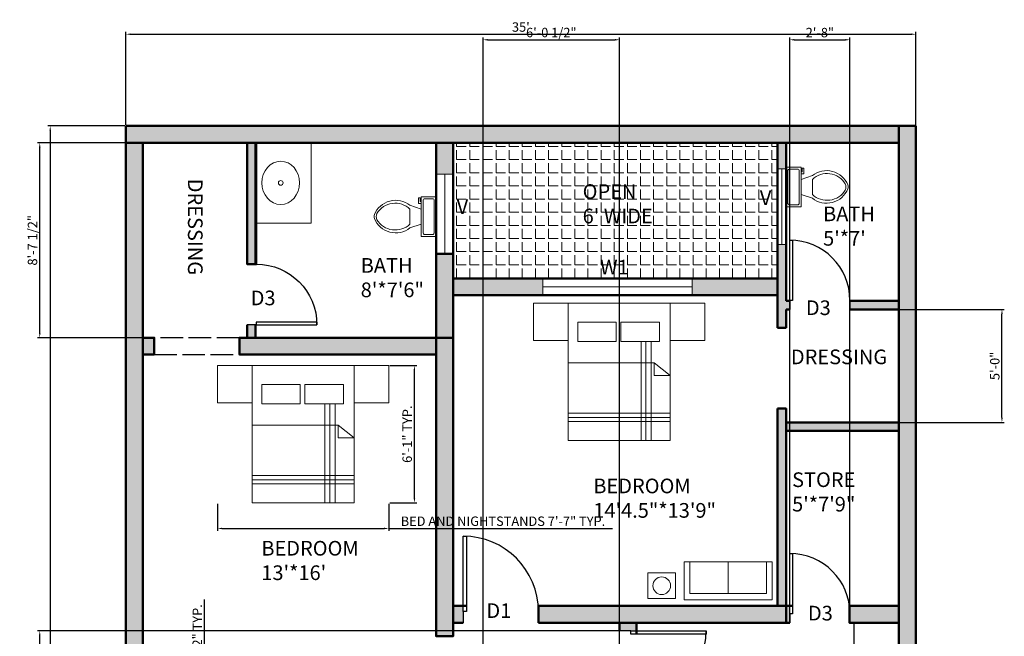
# Model space of a CAD drawing. Units: inches. Extents: x 2191 to 2715, y 2502 to 3448.
# Tile 3 of 3: x 2191 to 2715, y 3120 to 3448. Entities that reach past the tile are written whole.
import ezdxf

# ---------------------------------------------------------------- set-up
doc = ezdxf.new("R2010")
doc.units = ezdxf.units.IN
doc.linetypes.add('ACAD_ISO02W100', pattern=[15, 12, -3])
for name, color, linetype, lineweight in [('A-ANNO-DIMS', 2, 'Continuous', 18), ('A-AREA-IDEN', 130, 'Continuous', 25), ('A-FLOR-CASE', 9, 'Continuous', 25), ('A-FLOR-FIXT', 8, 'Continuous', 18), ('A-FLOR-PATT', 9, 'Continuous', 13), ('A-WALL-OVHD', 150, 'ACAD_ISO02W100', 25), ('A-WALL-PATT', 150, 'Continuous', 13), ('DOOR', 52, 'Continuous', 25), ('FUR', 140, 'Continuous', 18), ('TEXT', 130, 'Continuous', 18), ('WALL', 150, 'Continuous', 50), ('WIN', 210, 'Continuous', 18)]:
    doc.layers.add(name, color=color, linetype=linetype, lineweight=lineweight)
doc.styles.get("Standard").update_dxf_attribs({"font": 'arial.ttf'})
doc.dimstyles.new('ISO-25', dxfattribs={"dimtxt": 5, "dimasz": 2.5, "dimexe": 1.25, "dimexo": 0.625, "dimtad": 1, "dimdec": 0, "dimlunit": 4, "dimtxsty": 'Standard', "dimcen": 2.5, "dimadec": 0, "dimazin": 0, "dimtfac": 1, "dimtdec": 0, "dimtmove": 0, "dimatfit": 3, "dimfxl": 1, "dimarcsym": 0})

# ---------------------------------------------------------------- blocks, each defined once
blk = doc.blocks.new('*U2')
for p, q in [((0, 0), (0, -6)), ((40, 0), (40, -6))]:
    blk.add_line(p, q)
blk.add_lwpolyline([(0, 0), (0, 40), (1.75, 40), (1.75, 0)], close=True)
blk.add_arc((0, 0), 40, 0, 90)
blk = doc.blocks.new('*U4')
for p, q in [((9.5, -6), (9.5, -2)), ((-10, -8.5), (-8, -8.5)), ((-10, -9.5), (-10, -8.5)), ((-7, -9.5), (-10, -9.5)), ((-8, -8.5), (-8, -8)), ((-7, -8), (-7, -9.5)), ((-4, -8), (-6, -14)), ((4, -8), (6, -14)), ((4, -14), (-4, -14))]:
    blk.add_line(p, q)
blk.add_lwpolyline([(10.5, -8), (10.5, 0), (-10.5, 0), (-10.5, -8)], close=True)
for points in [[(-9.5, -2), (-9.5, -6)], [(8.5, -1), (-8.5, -1)], [(-8.5, -7), (8.5, -7)]]:
    blk.add_lwpolyline(points)
for centre, radius, start, end in [((-8.62, -1.88), 0.884, 81.8699, 188.1301), ((8.62, -1.88), 0.884, 351.8699, 98.1301), ((-8.62, -6.12), 0.884, 171.8699, 278.1301), ((8.62, -6.12), 0.884, 261.8699, 8.1301), ((3.52, -21.58), 12.17, 141.4691, 247.9714), ((4.2, -21.82), 11.33, 136.3677, 238.9468), ((-3.52, -21.58), 12.17, 292.0284, 38.5307), ((-4.2, -21.82), 11.33, 301.053, 43.6321), ((0, -27.88), 4, 245.7318, 294.2682), ((0, -29), 4, 254.8605, 285.1395)]:
    blk.add_arc(centre, radius, start, end)
blk = doc.blocks.new('*D8')
at = {"layer": 'A-ANNO-DIMS', "color": 0, "lineweight": -2, "transparency": 16777216}
for p, q in [((2247.96, 3392.28), (2247.96, 3441.65)), ((2250.46, 3440.4), (2665.46, 3440.4)), ((2667.96, 3392.28), (2667.96, 3441.65))]:
    blk.add_line(p, q, dxfattribs=at)
at = {"layer": 'A-ANNO-DIMS', "color": 0, "lineweight": 100, "transparency": 16777216}
for points in [[(2250.46, 3440.82), (2250.46, 3439.99), (2247.96, 3440.4)], [(2665.46, 3440.82), (2665.46, 3439.99), (2667.96, 3440.4)]]:
    blk.add_solid(points, dxfattribs=at)
at = {"layer": 'Defpoints', "color": 0, "lineweight": 100, "transparency": 16777216}
for p in [(2667.96, 3440.4), (2247.96, 3391.65), (2667.96, 3391.65)]:
    blk.add_point(p, dxfattribs=at)
at = {"layer": 'A-ANNO-DIMS', "color": 0, "transparency": 16777216, "insert": (2457.96, 3443.58), "char_height": 5, "attachment_point": 5}
blk.add_mtext("35'", dxfattribs=at)
blk = doc.blocks.new('*D9')
at = {"layer": 'A-ANNO-DIMS', "color": 0, "lineweight": -2, "transparency": 16777216}
for p, q in [((2247.34, 3391.65), (2206.49, 3391.65)), ((2207.74, 3389.15), (2207.74, 2554.15)), ((2247.34, 2551.65), (2206.49, 2551.65))]:
    blk.add_line(p, q, dxfattribs=at)
at = {"layer": 'A-ANNO-DIMS', "color": 0, "lineweight": 100, "transparency": 16777216}
for points in [[(2207.32, 3389.15), (2208.15, 3389.15), (2207.74, 3391.65)], [(2207.32, 2554.15), (2208.15, 2554.15), (2207.74, 2551.65)]]:
    blk.add_solid(points, dxfattribs=at)
at = {"layer": 'Defpoints', "color": 0, "lineweight": 100, "transparency": 16777216}
for p in [(2247.96, 3391.65), (2207.74, 2551.65), (2247.96, 2551.65)]:
    blk.add_point(p, dxfattribs=at)
at = {"layer": 'A-ANNO-DIMS', "color": 0, "transparency": 16777216, "insert": (2204.56, 2971.65), "char_height": 5, "attachment_point": 5, "rotation": 90}
blk.add_mtext("70'", dxfattribs=at)
blk = doc.blocks.new('BED-DOUBLE-WITH-NIGHTSTANDS')
for p, q in [((57.17, 52.58), (57.17, 0)), ((59.74, 52.58), (59.74, 0)), ((62.55, 52.58), (62.55, 0)), ((18.38, 41.27), (64.16, 41.27)), ((64.16, 41.27), (64.16, 34.46)), ((72.67, 34.46), (64.16, 41.27)), ((64.16, 34.46), (72.67, 34.46)), ((72.67, 14.44), (18.38, 14.44)), ((72.67, 12.22), (18.38, 12.22)), ((72.67, 10), (18.38, 10))]:
    blk.add_line(p, q)
for points in [[(0, 72.89), (18.38, 72.89), (18.38, 53.14), (0, 53.14)], [(18.38, 72.89), (72.67, 72.89), (72.67, 0), (18.38, 0)], [(72.67, 72.89), (91.05, 72.89), (91.05, 53.14), (72.67, 53.14)], [(46.51, 62.88), (66.93, 62.88), (66.93, 52.58), (46.51, 52.58)], [(23.55, 62.79), (43.97, 62.79), (43.97, 52.5), (23.55, 52.5)]]:
    blk.add_lwpolyline(points, close=True)
blk = doc.blocks.new('SOFA-TWO-SEAT')
for p, q in [((3.01, 20.24), (0, 20.24)), ((0, 20.24), (0, 0)), ((23.39, 20.24), (23.39, 3.45)), ((43.77, 20.24), (46.65, 20.24)), ((46.65, 20.24), (46.65, 20.24)), ((46.65, 20.24), (46.65, 0)), ((0, 0), (46.65, 0))]:
    blk.add_line(p, q)
blk.add_lwpolyline([(43.77, 3.45), (3.01, 3.45), (3.01, 20.24), (43.77, 20.24)], close=True)
blk = doc.blocks.new('TABLE-END-ROUND-ON-SQUARE')
blk.add_lwpolyline([(14.61, 0), (0, 0), (0, 13.55), (14.61, 13.55)], close=True)
blk.add_circle((7.31, 6.78), 4.68)
blk = doc.blocks.new('*D20')
at = {"layer": 'A-ANNO-DIMS', "color": 0, "lineweight": -2, "transparency": 16777216}
for p, q in [((2296.65, 3190.79), (2296.65, 3176.51)), ((2387.7, 3190.79), (2387.7, 3176.51)), ((2299.15, 3177.76), (2385.2, 3177.76)), ((2387.7, 3177.76), (2506.7, 3177.76))]:
    blk.add_line(p, q, dxfattribs=at)
at = {"layer": 'A-ANNO-DIMS', "color": 0, "lineweight": 100, "transparency": 16777216}
for points in [[(2299.15, 3178.17), (2299.15, 3177.34), (2296.65, 3177.76)], [(2385.2, 3178.17), (2385.2, 3177.34), (2387.7, 3177.76)]]:
    blk.add_solid(points, dxfattribs=at)
at = {"layer": 'Defpoints', "color": 0, "lineweight": 100, "transparency": 16777216}
for p in [(2296.65, 3191.41), (2387.7, 3191.41), (2387.7, 3177.76)]:
    blk.add_point(p, dxfattribs=at)
at = {"layer": 'A-ANNO-DIMS', "color": 0, "transparency": 16777216, "insert": (2448.45, 3180.97), "char_height": 5, "attachment_point": 5}
blk.add_mtext('BED AND NIGHTSTANDS 7\'-7" TYP.', dxfattribs=at)
blk = doc.blocks.new('*D21')
at = {"layer": 'A-ANNO-DIMS', "color": 0, "lineweight": -2, "transparency": 16777216}
for p, q in [((2388.33, 3264.3), (2402.61, 3264.3)), ((2401.36, 3193.91), (2401.36, 3261.8)), ((2388.33, 3191.41), (2402.61, 3191.41))]:
    blk.add_line(p, q, dxfattribs=at)
at = {"layer": 'A-ANNO-DIMS', "color": 0, "lineweight": 100, "transparency": 16777216}
for points in [[(2400.94, 3261.8), (2401.78, 3261.8), (2401.36, 3264.3)], [(2400.94, 3193.91), (2401.78, 3193.91), (2401.36, 3191.41)]]:
    blk.add_solid(points, dxfattribs=at)
at = {"layer": 'Defpoints', "color": 0, "lineweight": 100, "transparency": 16777216}
for p in [(2387.7, 3264.3), (2401.36, 3264.3), (2387.7, 3191.41)]:
    blk.add_point(p, dxfattribs=at)
at = {"layer": 'A-ANNO-DIMS', "color": 0, "transparency": 16777216, "insert": (2398.18, 3227.86), "char_height": 5, "attachment_point": 5, "rotation": 90}
blk.add_mtext('6\'-1" TYP.', dxfattribs=at)
blk = doc.blocks.new('*D26')
at = {"layer": 'A-ANNO-DIMS', "color": 0, "lineweight": -2, "transparency": 16777216}
for p, q in [((2289.77, 3038.86), (2289.77, 3139.97)), ((2298.34, 3038.86), (2288.52, 3038.86)), ((2289.77, 2980.06), (2289.77, 3036.36)), ((2298.34, 2977.56), (2288.52, 2977.56))]:
    blk.add_line(p, q, dxfattribs=at)
at = {"layer": 'A-ANNO-DIMS', "color": 0, "lineweight": 100, "transparency": 16777216}
for points in [[(2289.35, 3036.36), (2290.19, 3036.36), (2289.77, 3038.86)], [(2289.35, 2980.06), (2290.19, 2980.06), (2289.77, 2977.56)]]:
    blk.add_solid(points, dxfattribs=at)
at = {"layer": 'Defpoints', "color": 0, "lineweight": 100, "transparency": 16777216}
for p in [(2289.77, 3038.86), (2298.96, 3038.86), (2298.96, 2977.56)]:
    blk.add_point(p, dxfattribs=at)
at = {"layer": 'A-ANNO-DIMS', "color": 0, "transparency": 16777216, "insert": (2286.56, 3090.67), "char_height": 5, "attachment_point": 5, "rotation": 90}
blk.add_mtext('PATIO WINDOW 5\'-1 1/2" TYP.', dxfattribs=at)
blk = doc.blocks.new('*D28')
at = {"layer": 'A-ANNO-DIMS', "color": 0, "lineweight": -2, "transparency": 16777216}
for p, q in [((2509.84, 3123.41), (2200.91, 3123.41)), ((2202.16, 3085.91), (2202.16, 3120.91)), ((2509.84, 3083.41), (2200.91, 3083.41))]:
    blk.add_line(p, q, dxfattribs=at)
at = {"layer": 'A-ANNO-DIMS', "color": 0, "lineweight": 100, "transparency": 16777216}
for points in [[(2201.75, 3120.91), (2202.58, 3120.91), (2202.16, 3123.41)], [(2201.75, 3085.91), (2202.58, 3085.91), (2202.16, 3083.41)]]:
    blk.add_solid(points, dxfattribs=at)
at = {"layer": 'Defpoints', "color": 0, "lineweight": 100, "transparency": 16777216}
for p in [(2202.16, 3123.41), (2510.46, 3123.41), (2510.46, 3083.41)]:
    blk.add_point(p, dxfattribs=at)
at = {"layer": 'A-ANNO-DIMS', "color": 0, "transparency": 16777216, "insert": (2198.98, 3103.41), "char_height": 5, "attachment_point": 5, "rotation": 90}
blk.add_mtext('3\'-4"', dxfattribs=at)
blk = doc.blocks.new('*D29')
at = {"layer": 'A-ANNO-DIMS', "color": 0, "lineweight": -2, "transparency": 16777216}
for p, q in [((2600.93, 3128.28), (2600.93, 3438.7)), ((2603.43, 3437.45), (2630.45, 3437.45)), ((2632.95, 3128.28), (2632.95, 3438.7))]:
    blk.add_line(p, q, dxfattribs=at)
at = {"layer": 'A-ANNO-DIMS', "color": 0, "lineweight": 100, "transparency": 16777216}
for points in [[(2603.43, 3437.87), (2603.43, 3437.04), (2600.93, 3437.45)], [(2630.45, 3437.87), (2630.45, 3437.04), (2632.95, 3437.45)]]:
    blk.add_solid(points, dxfattribs=at)
at = {"layer": 'Defpoints', "color": 0, "lineweight": 100, "transparency": 16777216}
for p in [(2632.95, 3437.45), (2600.93, 3127.65), (2632.95, 3127.65)]:
    blk.add_point(p, dxfattribs=at)
at = {"layer": 'A-ANNO-DIMS', "color": 0, "transparency": 16777216, "insert": (2616.94, 3440.63), "char_height": 5, "attachment_point": 5}
blk.add_mtext('2\'-8"', dxfattribs=at)
blk = doc.blocks.new('*D33')
at = {"layer": 'A-ANNO-DIMS', "color": 0, "lineweight": -2, "transparency": 16777216}
for p, q in [((2437.84, 2847.78), (2437.84, 3438.7)), ((2440.34, 3437.45), (2507.96, 3437.45)), ((2510.46, 2847.78), (2510.46, 3438.7))]:
    blk.add_line(p, q, dxfattribs=at)
at = {"layer": 'A-ANNO-DIMS', "color": 0, "lineweight": 100, "transparency": 16777216}
for points in [[(2440.34, 3437.87), (2440.34, 3437.04), (2437.84, 3437.45)], [(2507.96, 3437.87), (2507.96, 3437.04), (2510.46, 3437.45)]]:
    blk.add_solid(points, dxfattribs=at)
at = {"layer": 'Defpoints', "color": 0, "lineweight": 100, "transparency": 16777216}
for p in [(2510.46, 3437.45), (2437.84, 2847.15), (2510.46, 2847.15)]:
    blk.add_point(p, dxfattribs=at)
at = {"layer": 'A-ANNO-DIMS', "color": 0, "transparency": 16777216, "insert": (2474.15, 3440.66), "char_height": 5, "attachment_point": 5}
blk.add_mtext('6\'-0 1/2"', dxfattribs=at)
blk = doc.blocks.new('*D38')
at = {"layer": 'A-ANNO-DIMS', "color": 0, "lineweight": -2, "transparency": 16777216}
for p, q in [((2659.59, 3294.15), (2715.01, 3294.15)), ((2713.76, 3236.65), (2713.76, 3291.65)), ((2659.59, 3234.15), (2715.01, 3234.15))]:
    blk.add_line(p, q, dxfattribs=at)
at = {"layer": 'A-ANNO-DIMS', "color": 0, "lineweight": 100, "transparency": 16777216}
for points in [[(2713.35, 3291.65), (2714.18, 3291.65), (2713.76, 3294.15)], [(2713.35, 3236.65), (2714.18, 3236.65), (2713.76, 3234.15)]]:
    blk.add_solid(points, dxfattribs=at)
at = {"layer": 'Defpoints', "color": 0, "lineweight": 100, "transparency": 16777216}
for p in [(2658.96, 3294.15), (2713.76, 3294.15), (2658.96, 3234.15)]:
    blk.add_point(p, dxfattribs=at)
at = {"layer": 'A-ANNO-DIMS', "color": 0, "transparency": 16777216, "insert": (2710.59, 3264.15), "char_height": 5, "attachment_point": 5, "rotation": 90}
blk.add_mtext('5\'-0"', dxfattribs=at)
blk = doc.blocks.new('*D39')
at = {"layer": 'A-ANNO-DIMS', "color": 0, "lineweight": -2, "transparency": 16777216}
for p, q in [((2256.34, 3382.65), (2200.91, 3382.65)), ((2202.16, 3281.65), (2202.16, 3380.15)), ((2256.34, 3279.15), (2200.91, 3279.15))]:
    blk.add_line(p, q, dxfattribs=at)
at = {"layer": 'A-ANNO-DIMS', "color": 0, "lineweight": 100, "transparency": 16777216}
for points in [[(2201.75, 3380.15), (2202.58, 3380.15), (2202.16, 3382.65)], [(2201.75, 3281.65), (2202.58, 3281.65), (2202.16, 3279.15)]]:
    blk.add_solid(points, dxfattribs=at)
at = {"layer": 'Defpoints', "color": 0, "lineweight": 100, "transparency": 16777216}
for p in [(2202.16, 3382.65), (2256.96, 3382.65), (2256.96, 3279.15)]:
    blk.add_point(p, dxfattribs=at)
at = {"layer": 'A-ANNO-DIMS', "color": 0, "transparency": 16777216, "insert": (2198.95, 3330.9), "char_height": 5, "attachment_point": 5, "rotation": 90}
blk.add_mtext('8\'-7 1/2"', dxfattribs=at)

msp = doc.modelspace()

# ---------------------------------------------------------------- hatches: boundary and pattern name
at = {"layer": 'A-FLOR-PATT'}
h = msp.add_hatch(dxfattribs=at)
h.set_pattern_fill('ANGLE', color=256)
h.set_pattern_definition([(0, (0, 0), (0, 6.985), [5.08, -1.905]), (90, (0, 0), (-6.985, 4e-16), [5.08, -1.905])])
h.paths.add_polyline_path([(2594.46, 3382.65), (2421.96, 3382.65), (2421.96, 3310.65), (2594.46, 3310.65)])
at = {"layer": 'A-WALL-PATT'}
h = msp.add_hatch(color=256, dxfattribs=at)
h.dxf.hatch_style = 1
h.paths.add_polyline_path([(2658.96, 3391.65), (2247.96, 3391.65), (2247.96, 3382.65), (2658.96, 3382.65)])
h.paths.add_polyline_path([(2256.96, 3382.65), (2247.96, 3382.65), (2247.96, 2561.19), (2256.96, 2561.19)])
h.paths.add_polyline_path([(2316.96, 3382.65), (2312.46, 3382.65), (2312.46, 3318.18), (2316.96, 3318.18)])
h.paths.add_polyline_path([(2412.96, 3279.15), (2308.33, 3279.15), (2308.33, 3270.15), (2412.96, 3270.15)])
h.paths.add_polyline_path([(2263, 3279.15), (2256.96, 3279.15), (2256.96, 3270.15), (2263, 3270.15)])
h.paths.add_polyline_path([(2421.96, 3323.7), (2412.96, 3323.7), (2412.96, 3279.15), (2421.96, 3279.15)])
h.paths.add_polyline_path([(2421.96, 3382.65), (2412.96, 3382.65), (2412.96, 3366.03), (2421.96, 3366.03)])
h.paths.add_polyline_path([(2421.96, 3279.15), (2412.96, 3279.15), (2412.96, 3270.15), (2412.96, 3120.46), (2421.96, 3120.46)])
h.paths.add_polyline_path([(2469.63, 3310.65), (2421.96, 3310.65), (2421.96, 3301.65), (2469.63, 3301.65)])
h.paths.add_polyline_path([(2594.46, 3310.65), (2549.09, 3310.65), (2549.09, 3301.65), (2594.46, 3301.65)])
h.paths.add_polyline_path([(2658.96, 3298.65), (2632.95, 3298.65), (2632.95, 3294.15), (2658.96, 3294.15)])
h.paths.add_polyline_path([(2600.93, 3298.65), (2598.96, 3298.65), (2598.96, 3328.67), (2594.46, 3328.67), (2594.46, 3310.65), (2594.46, 3294.15), (2594.46, 3284.36), (2598.96, 3284.36), (2598.96, 3294.15), (2600.93, 3294.15)])
h.paths.add_polyline_path([(2598.96, 3382.65), (2594.46, 3382.65), (2594.46, 3368.86), (2598.96, 3368.86), (2598.96, 3369.76)])
h.paths.add_polyline_path([(2667.96, 3391.65), (2658.96, 3391.65), (2658.96, 3382.65), (2658.96, 2551.65), (2667.96, 2551.65)])
h.paths.add_polyline_path([(2414.87, 2561.19), (2259.47, 2561.19), (2259.47, 2556.15), (2414.87, 2556.15)])
h.paths.add_polyline_path([(2259.47, 2561.19), (2247.96, 2561.19), (2247.96, 2551.65), (2259.47, 2551.65)])
h.paths.add_polyline_path([(2426.37, 2561.19), (2414.87, 2561.19), (2414.87, 2556.15), (2414.87, 2551.65), (2426.37, 2551.65), (2426.37, 2556.15)])
h.paths.add_polyline_path([(2667.96, 2556.15), (2426.37, 2556.15), (2426.37, 2551.65), (2667.96, 2551.65)])
h.paths.add_polyline_path([(2497.99, 2649.15), (2453.46, 2649.15), (2453.46, 2640.15), (2497.99, 2640.15)])
h.paths.add_polyline_path([(2462.96, 2693.64), (2453.46, 2693.64), (2453.46, 2649.15), (2462.96, 2649.15)])
h.paths.add_polyline_path([(2621.93, 2649.15), (2569.61, 2649.15), (2569.61, 2640.15), (2621.93, 2640.15)])
h.paths.add_polyline_path([(2610.96, 2721.15), (2606.46, 2721.15), (2606.46, 2649.15), (2610.96, 2649.15)])
h.paths.add_polyline_path([(2658.96, 2649.15), (2644.82, 2649.15), (2644.82, 2640.15), (2658.96, 2640.15)])
h.paths.add_polyline_path([(2462.96, 2784.15), (2453.46, 2784.15), (2453.46, 2733.49), (2459.46, 2733.49), (2462.96, 2733.49)])
h.paths.add_polyline_path([(2453.46, 2754.15), (2438.92, 2754.15), (2438.92, 2748.86), (2438.92, 2745.15), (2453.46, 2745.15)])
h.paths.add_polyline_path([(2389.52, 2754.15), (2256.96, 2754.15), (2256.96, 2745.15), (2389.52, 2745.15), (2389.52, 2748.86)])
h.paths.add_polyline_path([(2658.96, 2784.15), (2462.96, 2784.15), (2462.96, 2775.15), (2658.96, 2775.15)])
h.paths.add_polyline_path([(2658.96, 2725.65), (2639.65, 2725.65), (2639.65, 2721.68, -0.005), (2639.64, 2721.15), (2658.96, 2721.15)])
h.paths.add_polyline_path([(2613.17, 2725.65), (2606.46, 2725.65), (2606.46, 2721.15), (2610.96, 2721.15), (2613.17, 2721.15), (2613.17, 2721.68)])
h.paths.add_polyline_path([(2462.96, 2838.15), (2453.46, 2838.15), (2453.46, 2784.15), (2462.96, 2784.15)])
h.paths.add_polyline_path([(2389.52, 2847.15), (2256.96, 2847.15), (2256.96, 2838.15), (2389.52, 2838.15), (2389.52, 2841.86)])
h.paths.add_polyline_path([(2307.96, 2890.63), (2298.96, 2890.63), (2298.96, 2847.15), (2307.96, 2847.15)])
h.paths.add_polyline_path([(2462.96, 2847.15), (2453.96, 2847.15), (2438.92, 2847.15), (2438.92, 2841.86), (2438.92, 2838.15), (2453.96, 2838.15), (2462.96, 2838.15)])
h.paths.add_polyline_path([(2519.46, 2873.86, -0.01877), (2516.46, 2873.75), (2510.46, 2873.75), (2510.46, 2847.15), (2462.96, 2847.15), (2462.96, 2838.15), (2519.46, 2838.15)])
h.paths.add_polyline_path([(2519.46, 2922.15), (2510.46, 2922.15), (2510.46, 2913.75), (2516.46, 2913.75), (2519.46, 2913.75)])
h.paths.add_polyline_path([(2519.46, 2991.15), (2519.46, 3078.15), (2510.46, 3078.15), (2510.46, 3069.15), (2510.46, 2931.15), (2510.46, 2922.15), (2519.46, 2922.15), (2519.46, 2928.9), (2519.46, 2931.15)])
h.paths.add_polyline_path([(2609.08, 2926.65), (2556.08, 2926.65), (2556.08, 2922.15), (2609.08, 2922.15)])
h.paths.add_polyline_path([(2658.96, 2926.65), (2648.34, 2926.65), (2648.34, 2922.15), (2656.8, 2922.15), (2658.96, 2922.15)])
h.paths.add_polyline_path([(2603.46, 2931.15), (2603.46, 2935.9), (2598.96, 2935.9), (2598.96, 2931.15), (2598.96, 2926.65), (2603.46, 2926.65)])
h.paths.add_polyline_path([(2609.35, 3000.15), (2603.46, 3000.15), (2519.46, 3000.15), (2519.46, 2991.15), (2598.96, 2991.15), (2598.96, 2980.21), (2603.46, 2980.21), (2603.46, 2991.15), (2609.35, 2991.15)])
h.paths.add_polyline_path([(2658.96, 3000.15), (2649.75, 3000.15), (2649.75, 2991.15), (2658.96, 2991.15)])
h.paths.add_polyline_path([(2307.96, 2977.56), (2298.96, 2977.56), (2298.96, 2951.93), (2307.96, 2951.93)])
h.paths.add_polyline_path([(2307.96, 3069.15), (2298.96, 3069.15), (2298.96, 3038.86), (2307.96, 3038.86)])
h.paths.add_polyline_path([(2510.46, 3078.15), (2298.96, 3078.15), (2298.96, 3069.15), (2307.96, 3069.15), (2510.46, 3069.15)])
h.paths.add_polyline_path([(2421.96, 3080.46), (2415.96, 3080.46), (2412.96, 3080.46), (2412.96, 3078.15), (2421.96, 3078.15)])
h.paths.add_polyline_path([(2519.46, 3083.52, -0.01877), (2516.46, 3083.41), (2510.46, 3083.41), (2510.46, 3078.15), (2519.46, 3078.15)])
h.paths.add_polyline_path([(2519.46, 3127.65), (2510.46, 3127.65), (2510.46, 3123.41), (2516.46, 3123.41), (2519.46, 3123.41)])
h.paths.add_polyline_path([(2427.29, 3133.65), (2427.29, 3136.65), (2421.96, 3136.65), (2421.96, 3127.65), (2427.29, 3127.65)])
h.paths.add_polyline_path([(2598.96, 3136.65), (2467.29, 3136.65), (2467.29, 3127.65), (2598.96, 3127.65)])
h.paths.add_polyline_path([(2316.96, 3285.93), (2312.46, 3285.93), (2312.46, 3279.15), (2316.96, 3279.15)])
h.paths.add_polyline_path([(2658.96, 3234.15), (2598.96, 3234.15), (2598.96, 3229.65), (2658.96, 3229.65)])
h.paths.add_polyline_path([(2598.96, 3241.45), (2594.46, 3241.45), (2594.46, 3136.65), (2598.96, 3136.65)])
h.paths.add_polyline_path([(2658.96, 3136.65), (2632.67, 3136.65), (2632.67, 3127.65), (2658.96, 3127.65)])
h.paths.add_polyline_path([(2600.93, 3132.46), (2600.93, 3136.65), (2598.96, 3136.65), (2598.96, 3127.65), (2600.93, 3127.65)])
h.paths.add_polyline_path([(2524.07, 2926.65), (2519.46, 2926.65), (2519.46, 2922.15), (2524.07, 2922.15)])

# ---------------------------------------------------------------- linework, layer by layer
at = {"layer": 'A-FLOR-CASE'}
for p, q in [((2658.96, 3127.65), (2634.96, 3127.65)), ((2634.96, 3127.65), (2634.96, 3024.15))]:
    msp.add_line(p, q, dxfattribs=at)
at = {"layer": 'A-FLOR-FIXT'}
msp.add_lwpolyline([(2316.96, 3382.65), (2346.53, 3382.65), (2346.53, 3339.99), (2316.96, 3339.99)], close=True, dxfattribs=at)
msp.add_circle((2330.27, 3361.4), 1.25, dxfattribs=at)
msp.add_ellipse((2330.27, 3361.4), major_axis=(0, 11.49), ratio=0.872254, dxfattribs=at)
at = {"layer": 'A-WALL-OVHD'}
msp.add_lwpolyline([(2263, 3270.15), (2308.33, 3270.15), (2308.33, 3279.15), (2263, 3279.15)], close=True, dxfattribs=at)
at = {"layer": 'WALL'}
for p, q in [((2247.96, 3391.65), (2667.96, 3391.65)), ((2247.96, 2551.65), (2247.96, 3391.65)), ((2667.96, 3391.65), (2667.96, 2551.65)), ((2256.96, 3382.65), (2658.96, 3382.65)), ((2256.96, 2561.19), (2256.96, 3382.65)), ((2312.46, 3318.18), (2312.46, 3382.65)), ((2316.96, 3369.15), (2316.96, 3382.65)), ((2316.96, 3318.18), (2316.96, 3382.65)), ((2412.96, 3270.15), (2412.96, 3382.65)), ((2421.96, 3279.15), (2421.96, 3382.65)), ((2594.46, 3382.65), (2594.46, 3294.15)), ((2594.46, 3382.65), (2594.46, 3310.65)), ((2658.96, 3382.65), (2598.96, 3382.65)), ((2598.96, 3382.65), (2598.96, 3298.65)), ((2658.96, 3382.65), (2658.96, 2551.65)), ((2594.46, 3310.65), (2421.96, 3310.65)), ((2594.46, 3301.65), (2421.96, 3301.65)), ((2421.96, 3301.65), (2421.96, 3136.65)), ((2598.96, 3298.65), (2600.93, 3298.65)), ((2632.95, 3298.65), (2658.96, 3298.65)), ((2594.46, 3284.36), (2594.46, 3294.15)), ((2598.96, 3294.15), (2600.93, 3294.15)), ((2598.96, 3284.36), (2598.96, 3294.15)), ((2632.95, 3294.15), (2658.96, 3294.15)), ((2312.46, 3279.15), (2312.46, 3285.93)), ((2316.96, 3279.15), (2316.96, 3285.93)), ((2598.96, 3284.36), (2594.46, 3284.36)), ((2263, 3279.15), (2256.96, 3279.15)), ((2263, 3270.15), (2263, 3279.15)), ((2421.96, 3279.15), (2308.33, 3279.15)), ((2308.33, 3279.15), (2308.33, 3270.15)), ((2412.96, 3279.15), (2316.96, 3279.15)), ((2421.96, 3120.46), (2421.96, 3279.15)), ((2263, 3270.15), (2256.96, 3270.15)), ((2412.96, 3270.15), (2308.33, 3270.15)), ((2412.96, 3120.35), (2412.96, 3270.15)), ((2594.46, 3136.65), (2594.46, 3241.45)), ((2598.96, 3241.45), (2594.46, 3241.45)), ((2598.96, 3127.65), (2598.96, 3241.45)), ((2658.96, 3234.15), (2598.96, 3234.15)), ((2658.96, 3229.65), (2598.96, 3229.65)), ((2658.96, 3136.65), (2658.96, 3229.65)), ((2421.96, 3136.65), (2429.04, 3136.65)), ((2467.18, 3136.65), (2594.46, 3136.65)), ((2594.46, 3136.65), (2602.33, 3136.65)), ((2632.67, 3136.65), (2658.96, 3136.65)), ((2421.96, 3127.65), (2427.29, 3127.65)), ((2467.29, 3127.65), (2598.96, 3127.65)), ((2510.46, 3123.41), (2510.46, 3127.65)), ((2519.46, 3121.66), (2519.46, 3127.65)), ((2598.96, 3127.65), (2600.93, 3127.65)), ((2632.95, 3127.65), (2658.96, 3127.65))]:
    msp.add_line(p, q, dxfattribs=at)
for points in [[(2247.96, 3391.65), (2658.96, 3391.65), (2658.96, 3382.65), (2247.96, 3382.65)], [(2658.96, 3391.65), (2667.96, 3391.65), (2667.96, 2551.65), (2658.96, 2551.65)], [(2247.96, 2561.19), (2256.96, 2561.19), (2256.96, 3382.65), (2247.96, 3382.65)], [(2312.46, 3382.65), (2317.3, 3382.65), (2317.3, 3318.18), (2312.46, 3318.18)], [(2412.96, 3323.7), (2421.96, 3323.7), (2421.96, 3120.46), (2412.96, 3120.46)], [(2263, 3270.15), (2256.96, 3270.15), (2256.96, 3279.15), (2263, 3279.15)], [(2308.33, 3270.15), (2412.96, 3270.15), (2412.96, 3279.15), (2308.33, 3279.15)], [(2594.46, 3241.45), (2598.96, 3241.45), (2598.96, 3136.65), (2594.46, 3136.65)], [(2658.96, 3234.15), (2598.96, 3234.15), (2598.96, 3229.65), (2658.96, 3229.65)], [(2467.29, 3127.65), (2598.96, 3127.65), (2598.96, 3136.65), (2467.29, 3136.65)], [(2658.96, 3127.65), (2632.67, 3127.65), (2632.67, 3136.65), (2658.96, 3136.65)]]:
    msp.add_lwpolyline(points, close=True, dxfattribs=at)
at = {"layer": 'WIN'}
for p, q in [((2596.71, 3328.67), (2596.71, 3368.86)), ((2417.46, 3323.7), (2417.46, 3366.03)), ((2469.63, 3306.15), (2549.09, 3306.15))]:
    msp.add_line(p, q, dxfattribs=at)
for points in [[(2594.46, 3328.67), (2598.96, 3328.67), (2598.96, 3368.86), (2594.46, 3368.86)], [(2412.96, 3366.03), (2421.96, 3366.03), (2421.96, 3323.7), (2412.96, 3323.7)], [(2469.63, 3310.65), (2549.09, 3310.65), (2549.09, 3301.65), (2469.63, 3301.65)]]:
    msp.add_lwpolyline(points, close=True, dxfattribs=at)

# ---------------------------------------------------------------- block references
at = {"layer": 'A-FLOR-FIXT', "xscale": -1, "rotation": 90}
msp.add_blockref('*U4', (2598.96, 3359.26), dxfattribs=at)
at = {"layer": 'A-FLOR-FIXT', "rotation": 270}
msp.add_blockref('*U4', (2412.96, 3343.5), dxfattribs=at)
at = {"layer": 'DOOR', "xscale": 0.8003192358726801, "yscale": 0.8003192358726801, "zscale": 0.8003192358726801}
for p in [(2600.93, 3298.96), (2600.93, 3132.46)]:
    msp.add_blockref('*U2', p, dxfattribs=at)
at = {"layer": 'DOOR', "xscale": -0.8062553014010777, "yscale": 0.8062553014010777, "zscale": 0.8062553014010777, "rotation": 270}
msp.add_blockref('*U2', (2317.3, 3285.93), dxfattribs=at)
at = {"layer": 'DOOR'}
msp.add_blockref('*U2', (2427.29, 3133.65), dxfattribs=at)
at = {"layer": 'DOOR', "rotation": 270}
msp.add_blockref('*U2', (2516.46, 3123.41), dxfattribs=at)
at = {"layer": 'FUR'}
for name, p in [('BED-DOUBLE-WITH-NIGHTSTANDS', (2464.7, 3224.53)), ('BED-DOUBLE-WITH-NIGHTSTANDS', (2296.65, 3191.41)), ('SOFA-TWO-SEAT', (2544.87, 3139.82)), ('TABLE-END-ROUND-ON-SQUARE', (2525.56, 3140.55))]:
    msp.add_blockref(name, p, dxfattribs=at)

# ---------------------------------------------------------------- texts
at = {"layer": 'A-AREA-IDEN', "insert": (2288.76, 3363.58), "char_height": 7.795, "attachment_point": 1, "rotation": 270}
msp.add_mtext_dynamic_manual_height_columns('DRESSING', width=100.7314, gutter_width=38.97, heights=[0], dxfattribs=at)
at = {"layer": 'A-AREA-IDEN', "attachment_point": 1}
for s, insert, char_height in [("OPEN\\P6' WIDE", (2490.83, 3360.69), 7.795), ("BATH\\P5'*7'", (2618.67, 3348.84), 7.795), ('BATH\\P8\'*7\'6"', (2372.81, 3321.46), 7.795), ('DRESSING', (2601.55, 3272.84), 7.795), ('BEDROOM\\P14\'4.5"*13\'9"', (2496.5, 3204.25), 7.7945), ('STORE\\P5\'*7\'9"', (2602.19, 3207.57), 7.795), ("BEDROOM\\P13'*16'", (2319.99, 3171.14), 7.795)]:
    msp.add_mtext_dynamic_manual_height_columns(s, width=100.7314, gutter_width=38.97, heights=[0], dxfattribs=dict(at, insert=insert, char_height=char_height))
at = {"layer": 'TEXT', "attachment_point": 1}
for s, heights, insert, char_height in [('V', [0], (2585.03, 3357.39), 7.79), ('V', [0], (2423.83, 3352.66), 7.79), ('W1', [7.83], (2500.06, 3320.52), 7.795), ('D3', [0], (2314.32, 3304.15), 7.795), ('D3', [0], (2609.53, 3298.96), 7.795), ('D1', [0], (2439.66, 3137.98), 7.795), ('D3', [0], (2610.62, 3136.65), 7.795)]:
    msp.add_mtext_dynamic_manual_height_columns(s, width=100.7314, gutter_width=38.97, heights=heights, dxfattribs=dict(at, insert=insert, char_height=char_height))

# ---------------------------------------------------------------- dimensions: what is measured, and where the dimension line sits
at = {"layer": 'A-ANNO-DIMS'}
for base, p1, p2, override, picture, middle in [((2667.96, 3440.4), (2247.96, 3391.65), (2667.96, 3391.65), {"dimclrd": 0, "dimclre": 0, "dimclrt": 0}, '*D8', (2457.96, 3443.58)), ((2510.46, 3437.45), (2437.84, 2847.15), (2510.46, 2847.15), {"dimdec": 1, "dimlfac": 1, "dimrnd": 0, "dimzin": 1, "dimdsep": 46, "dimlunit": 4, "dimfrac": 2}, '*D33', (2474.15, 3440.66)), ((2632.95, 3437.45), (2600.93, 3127.65), (2632.95, 3127.65), {"dimdec": 1, "dimlfac": 1, "dimrnd": 0, "dimzin": 1, "dimdsep": 46, "dimlunit": 4, "dimfrac": 2}, '*D29', (2616.94, 3440.63))]:
    dim = msp.add_linear_dim(base=base, p1=p1, p2=p2, dimstyle='ISO-25', override=override, dxfattribs=at)
    dim.commit()
    dim.dimension.update_dxf_attribs({"geometry": picture, "text_midpoint": middle})
for base, p1, p2, override, picture, middle in [((2207.74, 2551.65), (2247.96, 3391.65), (2247.96, 2551.65), {"dimclrd": 0, "dimclre": 0, "dimclrt": 0}, '*D9', (2204.56, 2971.65)), ((2202.16, 3382.65), (2256.96, 3279.15), (2256.96, 3382.65), {"dimdec": 1, "dimlfac": 1, "dimrnd": 0, "dimzin": 1, "dimdsep": 46, "dimlunit": 4, "dimfrac": 2}, '*D39', (2198.95, 3330.9)), ((2713.76, 3294.15), (2658.96, 3234.15), (2658.96, 3294.15), {"dimdec": 1, "dimlfac": 1, "dimrnd": 0, "dimzin": 1, "dimdsep": 46, "dimlunit": 4, "dimfrac": 2}, '*D38', (2710.59, 3264.15)), ((2202.16, 3123.41), (2510.46, 3083.41), (2510.46, 3123.41), {"dimdec": 1, "dimlfac": 1, "dimrnd": 0, "dimzin": 1, "dimdsep": 46, "dimlunit": 4, "dimfrac": 2}, '*D28', (2198.98, 3103.41))]:
    dim = msp.add_linear_dim(base=base, p1=p1, p2=p2, angle=90, dimstyle='ISO-25', override=override, dxfattribs=at)
    dim.commit()
    dim.dimension.update_dxf_attribs({"geometry": picture, "text_midpoint": middle})
for base, p1, p2, text, picture, middle in [((2401.36, 3264.3), (2387.7, 3191.41), (2387.7, 3264.3), '<> TYP.', '*D21', (2398.18, 3227.86)), ((2289.77, 3038.86), (2298.96, 2977.56), (2298.96, 3038.86), 'PATIO WINDOW <> TYP.', '*D26', (2286.56, 3090.67))]:
    dim = msp.add_linear_dim(base=base, p1=p1, p2=p2, angle=90, text=text, dimstyle='ISO-25', override={"dimdec": 1, "dimlfac": 1, "dimrnd": 0, "dimzin": 1, "dimdsep": 46, "dimlunit": 4, "dimfrac": 2}, dxfattribs=at)
    dim.commit()
    dim.dimension.update_dxf_attribs({"geometry": picture, "text_midpoint": middle})
dim = msp.add_linear_dim(base=(2387.7012, 3177.7575), p1=(2296.6523, 3191.4148), p2=(2387.7012, 3191.4148), text='BED AND NIGHTSTANDS <> TYP.', dimstyle='ISO-25', override={"dimdec": 1, "dimlfac": 1, "dimrnd": 0, "dimzin": 1, "dimdsep": 46, "dimlunit": 4, "dimfrac": 2}, dxfattribs=at)
dim.commit()
dim.dimension.update_dxf_attribs({"geometry": '*D20', "text_midpoint": (2448.4507, 3180.9678)})

doc.saveas('drawing.dxf')
